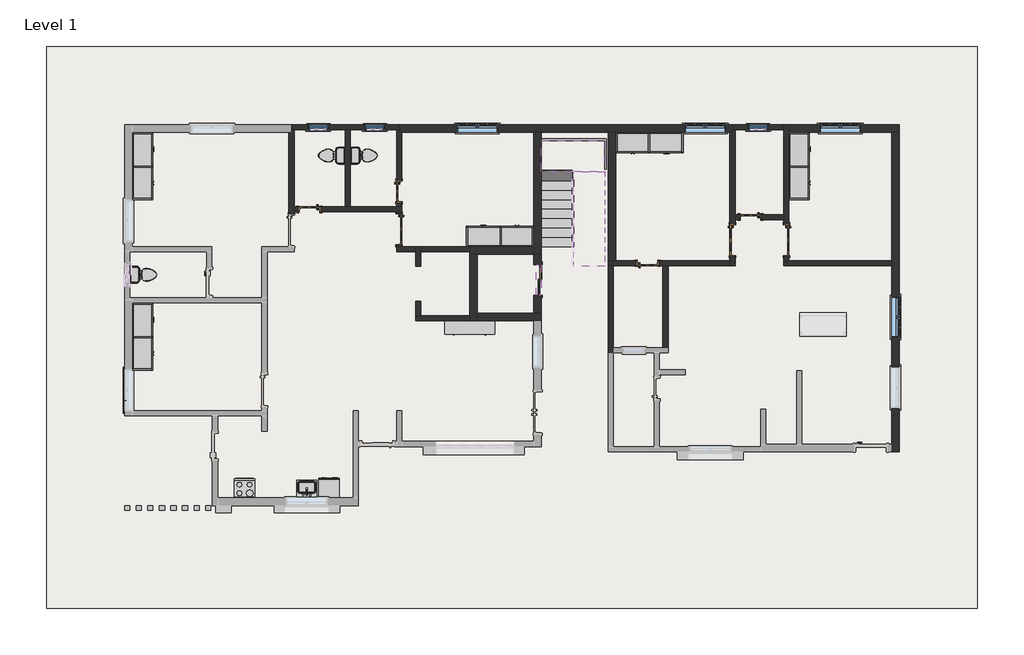
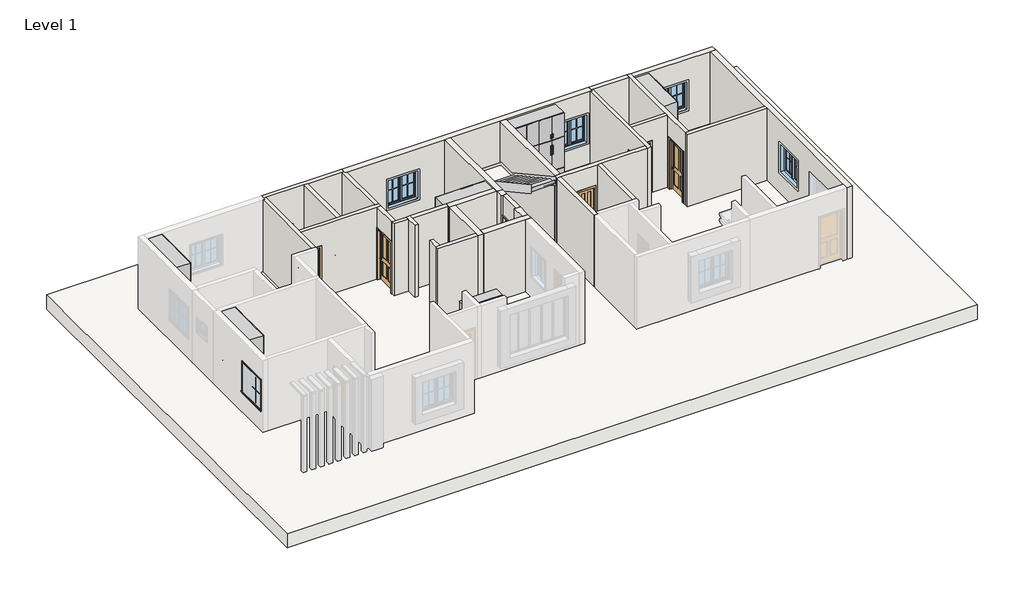
# One storey, part 2 of 3: 30 walls, 8 doors, 7 windows, 6 furniture elements, 4 flow terminals, 4 proxies, 2 slabs, 2 stair flights.
# Revit data of these elements (continued)
# Elements 47, 48, 49, 50, 51, 52, 53, 54, 55, 56 (IfcWall, "9\"") (continued)
#   Base Offset = 0' - 0"
#   wall height = 10' - 0"
#   Phase Created = New Construction
#   Base Constraint = Level 1
#   Top Constraint = Level 2
#   Materials on its faces: "wall"
# Element 57 (IfcWindow, "Window-Casement-Double : 4' X 4'")
#   Mark = "2"
#   Window Inset = 0' - 0"
#   Interior Wall Closure = 0' - 2 1/4"
#   Frame Extension = 0' - 0 1/4"
#   Exterior Wall Closure = 0' - 1 1/4"
#   Interior Trim Visibility = yes
#   Exterior Trim Visibility = yes
#   Phase Created = New Construction
#   Materials on its faces: "Wood - Stained", "Glass", "Clad - White"
# Element 58 (IfcWindow, "Window-Casement-Double : 4' X 4'")
#   Mark = "3"
#   Window Inset = 0' - 0"
#   Interior Wall Closure = 0' - 2 1/4"
#   Frame Extension = 0' - 0 1/4"
#   Exterior Wall Closure = 0' - 1 1/4"
#   Interior Trim Visibility = yes
#   Exterior Trim Visibility = yes
#   Phase Created = New Construction
#   Materials on its faces: "Wood - Stained", "Glass", "Clad - White"
# Element 59 (IfcWindow, "Window-Casement-Double : 4' X 4'")
#   Mark = "4"
#   Window Inset = 0' - 0"
#   Interior Wall Closure = 0' - 2 1/4"
#   Frame Extension = 0' - 0 1/4"
#   Exterior Wall Closure = 0' - 1 1/4"
#   Interior Trim Visibility = yes
#   Exterior Trim Visibility = yes
#   Phase Created = New Construction
#   Materials on its faces: "Wood - Stained", "Glass", "Clad - White"
# Element 60 (IfcWindow, "Window-Casement-Double : 4' X 4'")
#   Mark = "5"
#   Window Inset = 0' - 0"
#   Interior Wall Closure = 0' - 2 1/4"
#   Frame Extension = 0' - 0 1/4"
#   Exterior Wall Closure = 0' - 1 1/4"
#   Interior Trim Visibility = yes
#   Exterior Trim Visibility = yes
#   Phase Created = New Construction
#   Materials on its faces: "Wood - Stained", "Glass", "Clad - White"
# Element 61 (IfcWindow, "Window-Double-Hung : 2' X 2'")
#   Mark = "11"
#   Window Inset = 0' - 0"
#   Interior Wall Closure = 0' - 1 1/2"
#   Frame Extension = 0' - 1 1/4"
#   Exterior Wall Closure = 0' - 0 1/2"
#   Interior Trim Visibility = yes
#   Indicator Visibility = yes
#   Exterior Trim Visibility = yes
#   Phase Created = New Construction
#   Materials on its faces: "Wood - Stained", "Glass", "Clad - White"
# Element 62 (IfcWindow, "Window-Double-Hung : 2' X 2'")
#   Mark = "12"
#   Window Inset = 0' - 0"
#   Interior Wall Closure = 0' - 1 1/2"
#   Frame Extension = 0' - 1 1/4"
#   Exterior Wall Closure = 0' - 0 1/2"
#   Interior Trim Visibility = yes
#   Indicator Visibility = yes
#   Exterior Trim Visibility = yes
#   Phase Created = New Construction
#   Materials on its faces: "Wood - Stained", "Glass", "Clad - White"
# Element 63 (IfcWindow, "Window-Double-Hung : 2' X 2'")
#   Mark = "13"
#   Window Inset = 0' - 0"
#   Interior Wall Closure = 0' - 1 1/2"
#   Frame Extension = 0' - 1 1/4"
#   Exterior Wall Closure = 0' - 0 1/2"
#   Interior Trim Visibility = yes
#   Indicator Visibility = yes
#   Exterior Trim Visibility = yes
#   Phase Created = New Construction
#   Materials on its faces: "Wood - Stained", "Glass", "Clad - White"
# Materials
#   "Metal - Paint Finish - Ivory,Glossy": colour RGB 247 247 239, transparency 0
#   "Plastic - Black": colour RGB 0 0 0, transparency 0.7
#   "Metal - Chrome": class "Metal", colour RGB 17 17 17, transparency 0
#   "Metal - Painted Finish - Ivory,Matte": colour RGB 247 247 239, transparency 0
#   "Glass": class "Glass", colour RGB 0 128 192, transparency 0.75, Description = "Soda Lime Glass", Cost = 0
#   "Wood - Birch - Solid Stained Light Low Gloss": class "Wood", colour RGB 210 159 95, transparency 0, Cost = 0
#   "Paint - Sienna": colour RGB 118 70 51, transparency 0, Cost = 0
#   "Cherry": class "Wood", colour RGB 226 177 128, transparency 0, Description = "Prunus Serotina", Cost = 0
#   "Aluminum": class "Metal", colour RGB 247 247 247, transparency 0, Description = "Aluminum 6061", Cost = 0
#   "Metal - Steel, Polished": class "Metal", colour RGB 192 192 192, transparency 0
#   "Porcelain, Linen": class "Ceramic", colour RGB 249 239 230, transparency 0, Description = "Porcelain, linen", Cost = 0
#   "Laminate, Linen, Matte": class "Plastic", colour RGB 249 239 230, transparency 0, Description = "Plastic Laminate - Linen, Matte", Cost = 0
#   "Modern TV Stand - White Wood": class "Generic", colour RGB 120 120 120, transparency 0, Cost = 0
#   "Modern TV Stand - Semi Polished": class "Generic", colour RGB 120 120 120, transparency 0, Cost = 0
#   "Modern TV Stand - Oak Wood": class "Generic", colour RGB 120 120 120, transparency 0, Cost = 0
#   "FLOOR": class "Generic", colour RGB 189 255 255, transparency 0, Cost = 0
#   "wall": class "Generic", colour RGB 127 127 127, transparency 0, Cost = 0
#   "Wood - Stained": class "Wood", colour RGB 224 178 126, transparency 0, Cost = 0
#   "Clad - White": class "Wood", colour RGB 242 242 238, transparency 0, Cost = 0
#   "Phase - Demo": class "System", colour RGB 255 0 0, transparency 0.4, Cost = 0
#   "Default Wall": colour RGB 128 128 128, transparency 0, Cost = 0
#   "Phase - Exist": class "System", colour RGB 127 127 127, transparency 0, Cost = 0
#   "Default": colour RGB 127 127 127, transparency 0, Cost = 0
